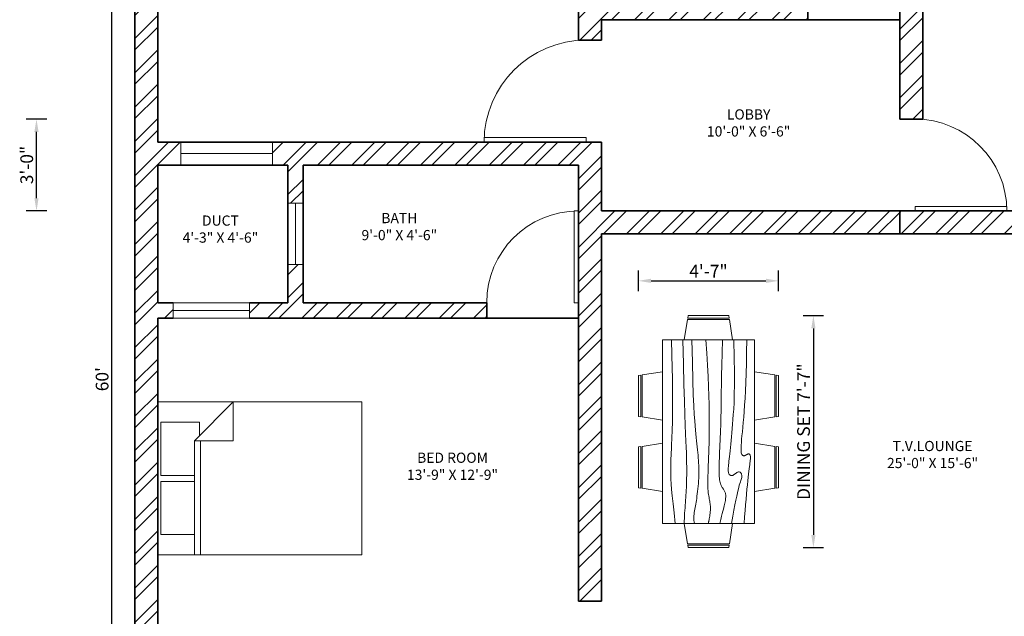
# Model space of a CAD drawing. Units: inches. Extents: x 468 to 1096, y 138 to 946.
# Tile 3 of 6: x 468 to 854, y 448 to 682. Entities that reach past the tile are written whole.
import ezdxf

# ---------------------------------------------------------------- set-up
doc = ezdxf.new("R2010")
doc.units = ezdxf.units.IN
doc.linetypes.add('ACAD_ISO02W100', pattern=[15, 12, -3])
for name, color, linetype, lineweight in [('A-ANNO-DIMS', 2, 'Continuous', 18), ('A-AREA-IDEN', 7, 'Continuous', 18), ('A-DOOR', 3, 'Continuous', 18), ('A-FURN', 8, 'Continuous', 18), ('A-GLAZ', 4, 'Continuous', 18), ('A-WALL', 7, 'Continuous', 35), ('A-WALL-OVHD', 7, 'ACAD_ISO02W100', 18), ('A-WALL-PATT', 8, 'Continuous', 13), ('C-PROP', 7, 'Continuous', 35)]:
    doc.layers.add(name, color=color, linetype=linetype, lineweight=lineweight)
doc.styles.get("Standard").update_dxf_attribs({"font": 'arial.ttf'})
doc.dimstyles.new('ISO-25', dxfattribs={"dimtxt": 5, "dimasz": 5, "dimexe": 4, "dimexo": 4, "dimtad": 1, "dimdec": 1, "dimlunit": 3, "dimtxsty": 'Standard', "dimcen": 2.5, "dimadec": 0, "dimazin": 0, "dimtfac": 1, "dimtdec": 1, "dimtmove": 0, "dimatfit": 3, "dimfxl": 4, "dimfxlon": 1, "dimarcsym": 0})

# ---------------------------------------------------------------- blocks, each defined once
blk = doc.blocks.new('*U2')
for p, q in [((0, 0), (0, -6)), ((40, 0), (40, -6))]:
    blk.add_line(p, q)
blk.add_lwpolyline([(0, 0), (0, 40), (1.75, 40), (1.75, 0)], close=True)
blk.add_arc((0, 0), 40, 0, 90)
blk = doc.blocks.new('*U3')
for p, q in [((0, 0), (0, -6)), ((-36, 0), (-36, -6))]:
    blk.add_line(p, q)
blk.add_lwpolyline([(0, 0), (0, 36), (-1.75, 36), (-1.75, 0)], close=True)
blk.add_arc((0, 0), 36, 90, 180)
blk = doc.blocks.new('Dining Set - 36 x 72 in.')
for p, q in [((-22, 27.5), (-22.1562, 26.50042)), ((-22, 27.5), (-6, 27.5)), ((-5.8437, 26.49966), (-6, 27.5)), ((6, 27.5), (5.8438, 26.50042)), ((6, 27.5), (22, 27.5)), ((22.1563, 26.49966), (22, 27.5)), ((-22.2343, 26.00059), (-23.4847, 17.99762)), ((-22.2304, 26), (-5.7608, 26)), ((-5.8416, 26.5), (-22.1534, 26.5)), ((-4.5152, 17.99762), (-5.7655, 25.99926)), ((5.7657, 26.00059), (4.5153, 17.99762)), ((5.7696, 26), (22.2392, 26)), ((22.1584, 26.5), (5.8466, 26.5)), ((23.4848, 17.99762), (22.2345, 25.99926)), ((36, 18), (-36, 18)), ((-36, 18), (-36, -18)), ((36, -18), (36, 18)), ((-45.5, 8), (-44.5004, 8.15617)), ((-45.5, 8), (-45.5, -8)), ((-44.5, -8.15843), (-44.5, 8.15338)), ((-44.0006, 8.23428), (-35.9976, 9.48474)), ((-44, 8.23041), (-44, -8.23915)), ((44.0006, 8.23428), (35.9976, 9.48474)), ((44, 8.23041), (44, -8.23915)), ((44.5, -8.15843), (44.5, 8.15338)), ((45.5, 8), (44.5005, 8.15617)), ((45.5, 8), (45.5, -8)), ((-44.4997, -8.15631), (-45.5, -8)), ((-35.9976, -9.48476), (-43.9993, -8.2345)), ((35.9976, -9.48476), (43.9993, -8.2345)), ((44.4997, -8.15631), (45.5, -8)), ((-36, -18), (36, -18)), ((-22.2343, -26.0006), (-23.4847, -17.99762)), ((-4.5152, -17.99762), (-5.7655, -25.99928)), ((5.7657, -26.0006), (4.5153, -17.99762)), ((23.4848, -17.99762), (22.2345, -25.99928)), ((-22.2304, -26), (-5.7608, -26)), ((-22, -27.5), (-22.1562, -26.50044)), ((-5.8416, -26.5), (-22.1534, -26.5)), ((-5.8437, -26.49967), (-6, -27.5)), ((5.7696, -26), (22.2392, -26)), ((6, -27.5), (5.8438, -26.50044)), ((22.1584, -26.5), (5.8466, -26.5)), ((22.1563, -26.49967), (22, -27.5)), ((-22, -27.5), (-6, -27.5)), ((6, -27.5), (22, -27.5))]:
    blk.add_line(p, q)
for points in [[(-36, 15), (-31.1772, 14.97754), (-26.8079, 14.91406), (-22.8538, 14.81543), (-19.276, 14.6875), (-16.0362, 14.53613), (-13.0957, 14.36718), (-10.4159, 14.18652), (-7.9583, 14), (-5.6904, 13.81315), (-3.6035, 13.63021), (-1.6954, 13.45508), (0.0365, 13.29166), (1.5945, 13.14388), (2.9811, 13.01562), (4.1988, 12.9108), (5.25, 12.83333), (6.1393, 12.78613), (6.8802, 12.76823), (7.4883, 12.77767), (7.9792, 12.8125), (8.3685, 12.87077), (8.6719, 12.95052), (8.9049, 13.0498), (9.0833, 13.16666), (9.2205, 13.29899), (9.3216, 13.44401), (9.3895, 13.59879), (9.4271, 13.76041), (9.4373, 13.92594), (9.4232, 14.09245), (9.3875, 14.257), (9.3333, 14.41666), (9.2638, 14.56917), (9.1836, 14.71484), (9.0975, 14.85465), (9.0104, 14.98958), (8.9272, 15.1206), (8.8529, 15.2487), (8.7922, 15.37483), (8.75, 15.5), (8.7305, 15.62467), (8.7344, 15.74739), (8.7617, 15.86621), (8.8125, 15.97916), (8.8867, 16.08431), (8.9844, 16.17968), (9.1055, 16.26334), (9.25, 16.33333), (9.4189, 16.38802), (9.6172, 16.42708), (9.8506, 16.45052), (10.125, 16.45833), (10.4463, 16.45052), (10.8203, 16.42708), (11.2529, 16.38802), (11.75, 16.33333), (12.3184, 16.26318), (12.9694, 16.17838), (13.7151, 16.07991), (14.5677, 15.96875), (15.5395, 15.84586), (16.6426, 15.71224), (17.8893, 15.56884), (19.2917, 15.41666), (20.859, 15.25667), (22.5879, 15.08984), (24.4721, 14.91715), (26.5052, 14.73958), (28.6809, 14.5581), (30.9929, 14.3737), (33.4347, 14.18733), (36, 14)], [(-36, 10), (-28.9766, 10.14274), (-23.1725, 10.20442), (-18.4241, 10.19775), (-14.5677, 10.13541), (-11.4399, 10.03011), (-8.877, 9.89453), (-6.7154, 9.74137), (-4.7917, 9.58333), (-2.9698, 9.43082), (-1.2246, 9.28515), (0.4415, 9.14534), (2.026, 9.01041), (3.5266, 8.87939), (4.9408, 8.7513), (6.266, 8.62516), (7.5, 8.5), (8.6411, 8.37549), (9.6914, 8.2539), (10.6538, 8.13818), (11.5312, 8.03125), (12.3267, 7.93603), (13.043, 7.85547), (13.6831, 7.79248), (14.25, 7.75), (14.7471, 7.7303), (15.1797, 7.73307), (15.5537, 7.75732), (15.875, 7.80208), (16.1494, 7.86637), (16.3828, 7.94922), (16.5811, 8.04964), (16.75, 8.16666), (16.8944, 8.29915), (17.0143, 8.44531), (17.1089, 8.60319), (17.1771, 8.77083), (17.218, 8.94629), (17.2305, 9.1276), (17.2137, 9.31282), (17.1667, 9.5), (17.0895, 9.6875), (16.987, 9.875), (16.8649, 10.0625), (16.7292, 10.25), (16.5856, 10.4375), (16.4401, 10.625), (16.2985, 10.8125), (16.1667, 11), (16.05, 11.18733), (15.9518, 11.3737), (15.8752, 11.5581), (15.8229, 11.73958), (15.798, 11.91715), (15.8034, 12.08984), (15.842, 12.25667), (15.9167, 12.41666), (16.0295, 12.56836), (16.1784, 12.70833), (16.3605, 12.83268), (16.5729, 12.9375), (16.8127, 13.01888), (17.0768, 13.07291), (17.3625, 13.0957), (17.6667, 13.08333), (17.9894, 13.03312), (18.3418, 12.94726), (18.7382, 12.82918), (19.1927, 12.68229), (19.7195, 12.51001), (20.3327, 12.31575), (21.0465, 12.10294), (21.875, 11.875), (22.8357, 11.63354), (23.959, 11.37304), (25.2786, 11.08618), (26.8282, 10.76562), (28.6414, 10.40405), (30.752, 9.99414), (33.1936, 9.52856), (36, 9)], [(-36, 5.5), (-30.7157, 5.3348), (-26.069, 5.20963), (-21.9946, 5.11767), (-18.4271, 5.05208), (-15.3009, 5.00602), (-12.5508, 4.97265), (-10.1112, 4.94515), (-7.9167, 4.91666), (-5.909, 4.88167), (-4.0586, 4.83984), (-2.3429, 4.79215), (-0.7396, 4.73958), (0.7739, 4.6831), (2.22, 4.6237), (3.6213, 4.56233), (5, 4.5), (6.373, 4.43782), (7.7344, 4.3776), (9.0723, 4.32129), (10.375, 4.27083), (11.6309, 4.22819), (12.8281, 4.19531), (13.9551, 4.17415), (15, 4.16666), (15.954, 4.17448), (16.819, 4.19791), (17.6001, 4.23698), (18.3021, 4.29166), (18.9299, 4.36198), (19.4883, 4.44791), (19.9823, 4.54948), (20.4167, 4.66666), (20.7969, 4.79899), (21.1302, 4.94401), (21.4245, 5.09879), (21.6875, 5.26041), (21.9271, 5.42594), (22.1511, 5.59245), (22.3672, 5.757), (22.5834, 5.91666), (22.8065, 6.06868), (23.0404, 6.21093), (23.2879, 6.34147), (23.5521, 6.45833), (23.8358, 6.55957), (24.142, 6.64323), (24.4735, 6.70735), (24.8334, 6.75), (25.2235, 6.76969), (25.642, 6.76692), (26.0858, 6.74267), (26.5521, 6.69791), (27.0379, 6.63362), (27.5404, 6.55078), (28.0565, 6.45036), (28.5834, 6.33333), (29.1242, 6.19987), (29.7071, 6.04687), (30.3661, 5.87044), (31.1354, 5.66666), (32.0493, 5.43164), (33.142, 5.16146), (34.4475, 4.85221), (36, 4.5)], [(-36, -1), (-30.7915, -0.6591), (-26.0195, -0.38216), (-21.6519, -0.16284), (-17.6563, 0.00521), (-14.0005, 0.12833), (-10.6523, 0.21289), (-7.5796, 0.26522), (-4.75, 0.29166), (-2.134, 0.29793), (0.2878, 0.28711), (2.5317, 0.26163), (4.6146, 0.22396), (6.5529, 0.17651), (8.3633, 0.12174), (10.0623, 0.06209), (11.6667, 0), (13.1899, -0.06201), (14.6341, -0.1211), (15.9982, -0.17432), (17.2813, -0.21875), (18.4823, -0.25147), (19.6003, -0.26953), (20.6343, -0.27002), (21.5834, -0.25), (22.4481, -0.20768), (23.2357, -0.14584), (23.9549, -0.06836), (24.6146, 0.02083), (25.2235, 0.11784), (25.7904, 0.21875), (26.3241, 0.31966), (26.8334, 0.41666), (27.3265, 0.50618), (27.8099, 0.58593), (28.2894, 0.65397), (28.7709, 0.70833), (29.2601, 0.74707), (29.763, 0.76823), (30.2855, 0.76985), (30.8334, 0.75), (31.4088, 0.70784), (31.9994, 0.64713), (32.589, 0.57275), (33.1615, 0.48958), (33.7008, 0.4025), (34.1908, 0.3164), (34.6153, 0.23616), (34.9584, 0.16666), (35.2099, 0.11165), (35.3848, 0.07031), (35.504, 0.04069), (35.5886, 0.02083), (35.6594, 0.00879), (35.7377, 0.0026), (35.8442, 0.00032), (36, 0)], [(-36, -6.5), (-27.1843, -6.31267), (-20.084, -6.1263), (-14.469, -5.9419), (-10.1094, -5.76042), (-6.7752, -5.58285), (-4.2363, -5.41016), (-2.2629, -5.24333), (-0.625, -5.08334), (0.8708, -4.93099), (2.2715, -4.78646), (3.5872, -4.64974), (4.8281, -4.52084), (6.0046, -4.39974), (7.127, -4.28646), (8.2053, -4.18099), (9.25, -4.08334), (10.2705, -3.99382), (11.2734, -3.91407), (12.2647, -3.84603), (13.25, -3.79167), (14.2354, -3.75293), (15.2266, -3.73177), (16.2295, -3.73015), (17.25, -3.75), (18.2912, -3.79248), (19.3451, -3.85547), (20.4009, -3.93604), (21.4479, -4.03125), (22.4754, -4.13819), (23.4727, -4.25391), (24.4289, -4.37549), (25.3334, -4.5), (26.1785, -4.62492), (26.9694, -4.74935), (27.7145, -4.87281), (28.4219, -4.99479), (29.1, -5.11483), (29.7572, -5.23242), (30.4016, -5.34709), (31.0417, -5.45834), (31.6837, -5.56437), (32.3262, -5.65821), (32.9658, -5.73153), (33.599, -5.77604), (34.2224, -5.78345), (34.8327, -5.74545), (35.4264, -5.65373), (36, -5.5)], [(-36, -10), (-26.4022, -9.81299), (-18.4675, -9.62891), (-11.9839, -9.45069), (-6.7396, -9.28125), (-2.5226, -9.12354), (0.8789, -8.98047), (3.6769, -8.85498), (6.0833, -8.75), (8.2767, -8.66765), (10.3021, -8.60677), (12.1712, -8.56543), (13.8958, -8.54167), (15.4876, -8.53353), (16.9583, -8.53907), (18.3197, -8.55632), (19.5834, -8.58334), (20.7616, -8.61841), (21.8685, -8.66081), (22.9188, -8.71004), (23.9271, -8.76563), (24.9081, -8.82707), (25.8763, -8.89388), (26.8465, -8.96558), (27.8334, -9.04167), (28.8474, -9.12118), (29.8828, -9.20117), (30.93, -9.27824), (31.9792, -9.34896), (33.0205, -9.40991), (34.0443, -9.45768), (35.0407, -9.48885), (36, -9.5)], [(-36, -14.5), (-30.0881, -14.33513), (-25.0332, -14.21224), (-20.7312, -14.12647), (-17.0781, -14.07292), (-13.97, -14.04671), (-11.3027, -14.04297), (-8.9724, -14.05681), (-6.875, -14.08334), (-4.9224, -14.11833), (-3.0905, -14.16016), (-1.3709, -14.20785), (0.2448, -14.26042), (1.7647, -14.3169), (3.1973, -14.3763), (4.5507, -14.43767), (5.8333, -14.5), (7.0554, -14.5621), (8.235, -14.62175), (9.3922, -14.67652), (10.5469, -14.72396), (11.7192, -14.76164), (12.929, -14.78711), (14.1965, -14.79794), (15.5417, -14.79167), (16.9933, -14.76424), (18.6152, -14.70508), (20.4804, -14.60197), (22.6615, -14.44271), (25.2312, -14.21509), (28.2624, -13.9069), (31.8277, -13.50594), (36, -13)]]:
    blk.add_lwpolyline(points)
blk = doc.blocks.new('Bed - Queen')
for p, q in [((0, -80.00003), (0, 0)), ((0, 0), (59.99999, 0)), ((59.99999, 0), (59.99999, -80.00003)), ((7.99999, -1.2), (28.79998, -1.2)), ((7.99999, -14.4), (7.99999, -1.2)), ((28.79998, -1.2), (28.79998, -14.4)), ((31.19999, -1.2), (51.99999, -1.2)), ((31.19999, -14.4), (31.19999, -1.2)), ((51.99999, -1.2), (51.99999, -16.4)), ((0, -14.4), (44.8, -14.4)), ((59.99999, -29.6), (44.8, -14.4)), ((44.8, -14.4), (44.8, -29.6)), ((44.8, -16.8), (0, -16.8)), ((51.99999, -16.4), (46.79936, -16.4)), ((44.8, -29.6), (59.99999, -29.6)), ((59.99999, -80.00003), (0, -80.00003))]:
    blk.add_line(p, q)
blk = doc.blocks.new('*D18')
at = {"layer": 'A-ANNO-DIMS', "color": 0, "lineweight": -2, "transparency": 16777216}
for p, q in [((508.14, 901.16), (500.14, 901.16)), ((504.14, 186.16), (504.14, 896.16)), ((508.14, 181.16), (500.14, 181.16))]:
    blk.add_line(p, q, dxfattribs=at)
at = {"layer": 'A-ANNO-DIMS', "color": 0, "transparency": 16777216}
for points in [[(503.3, 896.16), (504.97, 896.16), (504.14, 901.16)], [(503.3, 186.16), (504.97, 186.16), (504.14, 181.16)]]:
    blk.add_solid(points, dxfattribs=at)
at = {"layer": 'Defpoints', "color": 0, "transparency": 16777216}
for p in [(504.14, 901.16), (513.13, 901.16), (513.13, 181.16)]:
    blk.add_point(p, dxfattribs=at)
at = {"layer": 'A-ANNO-DIMS', "color": 0, "transparency": 16777216, "insert": (500.96, 541.16), "char_height": 5, "attachment_point": 5, "rotation": 90}
blk.add_mtext("60'", dxfattribs=at)
blk = doc.blocks.new('WIN-36-W9')
for p, q in [((0, 9), (0, 0)), ((36, 9), (36, 0)), ((0, 4.5), (36, 4.5))]:
    blk.add_line(p, q)
blk = doc.blocks.new('*D47')
at = {"layer": 'A-ANNO-DIMS', "color": 0, "lineweight": -2, "transparency": 16777216}
for p, q in [((775.26, 566.09), (783.26, 566.09)), ((779.26, 561.09), (779.26, 480.09)), ((775.26, 475.09), (783.26, 475.09))]:
    blk.add_line(p, q, dxfattribs=at)
at = {"layer": 'A-ANNO-DIMS', "color": 0, "transparency": 16777216}
for points in [[(778.42, 561.09), (780.09, 561.09), (779.26, 566.09)], [(778.42, 480.09), (780.09, 480.09), (779.26, 475.09)]]:
    blk.add_solid(points, dxfattribs=at)
at = {"layer": 'Defpoints', "color": 0, "transparency": 16777216}
for p in [(765.61, 566.09), (765.61, 475.09), (779.26, 475.09)]:
    blk.add_point(p, dxfattribs=at)
at = {"layer": 'A-ANNO-DIMS', "color": 0, "transparency": 16777216, "insert": (776.05, 520.59), "char_height": 5, "attachment_point": 5, "rotation": 90}
blk.add_mtext('DINING SET 7\'-7"', dxfattribs=at)
blk = doc.blocks.new('*D48')
at = {"layer": 'A-ANNO-DIMS', "color": 0, "lineweight": -2, "transparency": 16777216}
for p, q in [((710.61, 575.74), (710.61, 583.74)), ((765.61, 575.74), (765.61, 583.74)), ((715.61, 579.74), (760.61, 579.74))]:
    blk.add_line(p, q, dxfattribs=at)
at = {"layer": 'A-ANNO-DIMS', "color": 0, "transparency": 16777216}
for points in [[(715.61, 580.57), (715.61, 578.91), (710.61, 579.74)], [(760.61, 580.57), (760.61, 578.91), (765.61, 579.74)]]:
    blk.add_solid(points, dxfattribs=at)
at = {"layer": 'Defpoints', "color": 0, "transparency": 16777216}
for p in [(765.61, 579.74), (710.61, 566.09), (765.61, 566.09)]:
    blk.add_point(p, dxfattribs=at)
at = {"layer": 'A-ANNO-DIMS', "color": 0, "transparency": 16777216, "insert": (738.11, 582.87), "char_height": 5, "attachment_point": 5}
blk.add_mtext('4\'-7"', dxfattribs=at)
blk = doc.blocks.new('*D61')
at = {"layer": 'A-ANNO-DIMS', "color": 0, "lineweight": -2, "transparency": 16777216}
for p, q in [((594.13, 146.61), (594.13, 138.61)), ((630.13, 146.61), (630.13, 138.61)), ((599.13, 142.61), (625.13, 142.61))]:
    blk.add_line(p, q, dxfattribs=at)
at = {"layer": 'A-ANNO-DIMS', "color": 0, "transparency": 16777216}
for points in [[(599.13, 143.44), (599.13, 141.78), (594.13, 142.61)], [(625.13, 143.44), (625.13, 141.78), (630.13, 142.61)]]:
    blk.add_solid(points, dxfattribs=at)
at = {"layer": 'Defpoints', "color": 0, "transparency": 16777216}
for p in [(594.13, 829.16), (630.13, 826.16), (630.13, 142.61)]:
    blk.add_point(p, dxfattribs=at)
at = {"layer": 'A-ANNO-DIMS', "color": 0, "transparency": 16777216, "insert": (612.13, 145.79), "char_height": 5, "attachment_point": 5}
blk.add_mtext('3\'-0"', dxfattribs=at)
blk = doc.blocks.new('*D63')
at = {"layer": 'A-ANNO-DIMS', "color": 0, "lineweight": -2, "transparency": 16777216}
for p, q in [((777.13, 146.61), (777.13, 138.61)), ((813.13, 146.61), (813.13, 138.61)), ((782.13, 142.61), (808.13, 142.61))]:
    blk.add_line(p, q, dxfattribs=at)
at = {"layer": 'A-ANNO-DIMS', "color": 0, "transparency": 16777216}
for points in [[(782.13, 143.44), (782.13, 141.78), (777.13, 142.61)], [(808.13, 143.44), (808.13, 141.78), (813.13, 142.61)]]:
    blk.add_solid(points, dxfattribs=at)
at = {"layer": 'Defpoints', "color": 0, "transparency": 16777216}
for p in [(777.13, 682.16), (813.13, 682.16), (813.13, 142.61)]:
    blk.add_point(p, dxfattribs=at)
at = {"layer": 'A-ANNO-DIMS', "color": 0, "transparency": 16777216, "insert": (795.13, 145.79), "char_height": 5, "attachment_point": 5}
blk.add_mtext('3\'-0"', dxfattribs=at)
blk = doc.blocks.new('*D66')
at = {"layer": 'A-ANNO-DIMS', "color": 0, "lineweight": -2, "transparency": 16777216}
for p, q in [((696.13, 146.61), (696.13, 138.61)), ((714.39, 146.61), (714.39, 138.61)), ((701.13, 142.61), (709.39, 142.61)), ((714.39, 142.61), (745.11, 142.61))]:
    blk.add_line(p, q, dxfattribs=at)
at = {"layer": 'A-ANNO-DIMS', "color": 0, "transparency": 16777216}
for points in [[(701.13, 143.44), (701.13, 141.78), (696.13, 142.61)], [(709.39, 143.44), (709.39, 141.78), (714.39, 142.61)]]:
    blk.add_solid(points, dxfattribs=at)
at = {"layer": 'Defpoints', "color": 0, "transparency": 16777216}
for p in [(696.13, 820.16), (714.39, 802.16), (714.39, 142.61)]:
    blk.add_point(p, dxfattribs=at)
at = {"layer": 'A-ANNO-DIMS', "color": 0, "transparency": 16777216, "insert": (732.25, 145.82), "char_height": 5, "attachment_point": 5}
blk.add_mtext('1\'-6 1/2"', dxfattribs=at)
blk = doc.blocks.new('*D75')
at = {"layer": 'A-ANNO-DIMS', "color": 0, "lineweight": -2, "transparency": 16777216}
for p, q in [((696.13, 935.71), (696.13, 943.71)), ((736.13, 935.71), (736.13, 943.71)), ((701.13, 939.71), (731.13, 939.71))]:
    blk.add_line(p, q, dxfattribs=at)
at = {"layer": 'A-ANNO-DIMS', "color": 0, "transparency": 16777216}
for points in [[(701.13, 940.54), (701.13, 938.88), (696.13, 939.71)], [(731.13, 940.54), (731.13, 938.88), (736.13, 939.71)]]:
    blk.add_solid(points, dxfattribs=at)
at = {"layer": 'Defpoints', "color": 0, "transparency": 16777216}
for p in [(736.13, 939.71), (696.13, 412.16), (736.13, 412.16)]:
    blk.add_point(p, dxfattribs=at)
at = {"layer": 'A-ANNO-DIMS', "color": 0, "transparency": 16777216, "insert": (716.13, 942.89), "char_height": 5, "attachment_point": 5}
blk.add_mtext('3\'-4"', dxfattribs=at)
blk = doc.blocks.new('*D76')
at = {"layer": 'A-ANNO-DIMS', "color": 0, "lineweight": -2, "transparency": 16777216}
for p, q in [((1087.68, 454.16), (1095.68, 454.16)), ((1091.68, 423.16), (1091.68, 449.16)), ((1087.68, 418.16), (1095.68, 418.16))]:
    blk.add_line(p, q, dxfattribs=at)
at = {"layer": 'A-ANNO-DIMS', "color": 0, "transparency": 16777216}
for points in [[(1090.85, 449.16), (1092.51, 449.16), (1091.68, 454.16)], [(1090.85, 423.16), (1092.51, 423.16), (1091.68, 418.16)]]:
    blk.add_solid(points, dxfattribs=at)
at = {"layer": 'Defpoints', "color": 0, "transparency": 16777216}
for p in [(687.13, 454.16), (1091.68, 454.16), (687.13, 418.16)]:
    blk.add_point(p, dxfattribs=at)
at = {"layer": 'A-ANNO-DIMS', "color": 0, "transparency": 16777216, "insert": (1088.5, 436.16), "char_height": 5, "attachment_point": 5, "rotation": 90}
blk.add_mtext('3\'-0"', dxfattribs=at)
blk = doc.blocks.new('*D77')
at = {"layer": 'A-ANNO-DIMS', "color": 0, "lineweight": -2, "transparency": 16777216}
for p, q in [((651.13, 146.61), (651.13, 138.61)), ((687.13, 146.61), (687.13, 138.61)), ((656.13, 142.61), (682.13, 142.61))]:
    blk.add_line(p, q, dxfattribs=at)
at = {"layer": 'A-ANNO-DIMS', "color": 0, "transparency": 16777216}
for points in [[(656.13, 143.44), (656.13, 141.78), (651.13, 142.61)], [(682.13, 143.44), (682.13, 141.78), (687.13, 142.61)]]:
    blk.add_solid(points, dxfattribs=at)
at = {"layer": 'Defpoints', "color": 0, "transparency": 16777216}
for p in [(651.13, 565.16), (687.13, 565.16), (687.13, 142.61)]:
    blk.add_point(p, dxfattribs=at)
at = {"layer": 'A-ANNO-DIMS', "color": 0, "transparency": 16777216, "insert": (669.13, 145.79), "char_height": 5, "attachment_point": 5}
blk.add_mtext('3\'-0"', dxfattribs=at)
blk = doc.blocks.new('*D78')
at = {"layer": 'A-ANNO-DIMS', "color": 0, "lineweight": -2, "transparency": 16777216}
for p, q in [((573.13, 935.71), (573.13, 943.71)), ((603.13, 935.71), (603.13, 943.71)), ((578.13, 939.71), (598.13, 939.71))]:
    blk.add_line(p, q, dxfattribs=at)
at = {"layer": 'A-ANNO-DIMS', "color": 0, "transparency": 16777216}
for points in [[(578.13, 940.54), (578.13, 938.88), (573.13, 939.71)], [(598.13, 940.54), (598.13, 938.88), (603.13, 939.71)]]:
    blk.add_solid(points, dxfattribs=at)
at = {"layer": 'Defpoints', "color": 0, "transparency": 16777216}
for p in [(603.13, 939.71), (573.13, 250.16), (603.13, 250.16)]:
    blk.add_point(p, dxfattribs=at)
at = {"layer": 'A-ANNO-DIMS', "color": 0, "transparency": 16777216, "insert": (588.13, 942.89), "char_height": 5, "attachment_point": 5}
blk.add_mtext('2\'-6"', dxfattribs=at)
blk = doc.blocks.new('*D79')
at = {"layer": 'A-ANNO-DIMS', "color": 0, "lineweight": -2, "transparency": 16777216}
for p, q in [((612.13, 935.71), (612.13, 943.71)), ((636.13, 935.71), (636.13, 943.71)), ((617.13, 939.71), (631.13, 939.71))]:
    blk.add_line(p, q, dxfattribs=at)
at = {"layer": 'A-ANNO-DIMS', "color": 0, "transparency": 16777216}
for points in [[(617.13, 940.54), (617.13, 938.88), (612.13, 939.71)], [(631.13, 940.54), (631.13, 938.88), (636.13, 939.71)]]:
    blk.add_solid(points, dxfattribs=at)
at = {"layer": 'Defpoints', "color": 0, "transparency": 16777216}
for p in [(636.13, 939.71), (612.13, 241.16), (636.13, 241.16)]:
    blk.add_point(p, dxfattribs=at)
at = {"layer": 'A-ANNO-DIMS', "color": 0, "transparency": 16777216, "insert": (624.13, 942.89), "char_height": 5, "attachment_point": 5}
blk.add_mtext('2\'-0"', dxfattribs=at)
blk = doc.blocks.new('*D80')
at = {"layer": 'A-ANNO-DIMS', "color": 0, "lineweight": -2, "transparency": 16777216}
for p, q in [((684.13, 935.71), (684.13, 943.71)), ((708.13, 935.71), (708.13, 943.71)), ((689.13, 939.71), (703.13, 939.71))]:
    blk.add_line(p, q, dxfattribs=at)
at = {"layer": 'A-ANNO-DIMS', "color": 0, "transparency": 16777216}
for points in [[(689.13, 940.54), (689.13, 938.88), (684.13, 939.71)], [(703.13, 940.54), (703.13, 938.88), (708.13, 939.71)]]:
    blk.add_solid(points, dxfattribs=at)
at = {"layer": 'Defpoints', "color": 0, "transparency": 16777216}
for p in [(708.13, 939.71), (684.13, 250.16), (708.13, 250.16)]:
    blk.add_point(p, dxfattribs=at)
at = {"layer": 'A-ANNO-DIMS', "color": 0, "transparency": 16777216, "insert": (696.13, 942.89), "char_height": 5, "attachment_point": 5}
blk.add_mtext('2\'-0"', dxfattribs=at)
blk = doc.blocks.new('*D81')
at = {"layer": 'A-ANNO-DIMS', "color": 0, "lineweight": -2, "transparency": 16777216}
for p, q in [((708.13, 935.71), (708.13, 943.71)), ((744.13, 935.71), (744.13, 943.71)), ((713.13, 939.71), (739.13, 939.71))]:
    blk.add_line(p, q, dxfattribs=at)
at = {"layer": 'A-ANNO-DIMS', "color": 0, "transparency": 16777216}
for points in [[(713.13, 940.54), (713.13, 938.88), (708.13, 939.71)], [(739.13, 940.54), (739.13, 938.88), (744.13, 939.71)]]:
    blk.add_solid(points, dxfattribs=at)
at = {"layer": 'Defpoints', "color": 0, "transparency": 16777216}
for p in [(744.13, 939.71), (708.13, 250.16), (744.13, 250.16)]:
    blk.add_point(p, dxfattribs=at)
at = {"layer": 'A-ANNO-DIMS', "color": 0, "transparency": 16777216, "insert": (726.13, 942.89), "char_height": 5, "attachment_point": 5}
blk.add_mtext('3\'-0"', dxfattribs=at)
blk = doc.blocks.new('*D82')
at = {"layer": 'A-ANNO-DIMS', "color": 0, "lineweight": -2, "transparency": 16777216}
for p, q in [((1087.68, 674.16), (1095.68, 674.16)), ((1091.68, 639.16), (1091.68, 669.16)), ((1087.68, 634.16), (1095.68, 634.16))]:
    blk.add_line(p, q, dxfattribs=at)
at = {"layer": 'A-ANNO-DIMS', "color": 0, "transparency": 16777216}
for points in [[(1090.85, 669.16), (1092.51, 669.16), (1091.68, 674.16)], [(1090.85, 639.16), (1092.51, 639.16), (1091.68, 634.16)]]:
    blk.add_solid(points, dxfattribs=at)
at = {"layer": 'Defpoints', "color": 0, "transparency": 16777216}
for p in [(687.13, 674.16), (1091.68, 674.16), (687.13, 634.16)]:
    blk.add_point(p, dxfattribs=at)
at = {"layer": 'A-ANNO-DIMS', "color": 0, "transparency": 16777216, "insert": (1088.5, 654.16), "char_height": 5, "attachment_point": 5, "rotation": 90}
blk.add_mtext('3\'-4"', dxfattribs=at)
blk = doc.blocks.new('*D83')
at = {"layer": 'A-ANNO-DIMS', "color": 0, "lineweight": -2, "transparency": 16777216}
for p, q in [((478.58, 643.16), (470.58, 643.16)), ((474.58, 612.16), (474.58, 638.16)), ((478.58, 607.16), (470.58, 607.16))]:
    blk.add_line(p, q, dxfattribs=at)
at = {"layer": 'A-ANNO-DIMS', "color": 0, "transparency": 16777216}
for points in [[(473.75, 638.16), (475.41, 638.16), (474.58, 643.16)], [(473.75, 612.16), (475.41, 612.16), (474.58, 607.16)]]:
    blk.add_solid(points, dxfattribs=at)
at = {"layer": 'Defpoints', "color": 0, "transparency": 16777216}
for p in [(474.58, 643.16), (813.13, 643.16), (813.13, 607.16)]:
    blk.add_point(p, dxfattribs=at)
at = {"layer": 'A-ANNO-DIMS', "color": 0, "transparency": 16777216, "insert": (471.4, 625.16), "char_height": 5, "attachment_point": 5, "rotation": 90}
blk.add_mtext('3\'-0"', dxfattribs=at)
blk = doc.blocks.new('*D85')
at = {"layer": 'A-ANNO-DIMS', "color": 0, "lineweight": -2, "transparency": 16777216}
for p, q in [((528.13, 146.61), (528.13, 138.61)), ((558.13, 146.61), (558.13, 138.61)), ((533.13, 142.61), (553.13, 142.61))]:
    blk.add_line(p, q, dxfattribs=at)
at = {"layer": 'A-ANNO-DIMS', "color": 0, "transparency": 16777216}
for points in [[(533.13, 143.44), (533.13, 141.78), (528.13, 142.61)], [(553.13, 143.44), (553.13, 141.78), (558.13, 142.61)]]:
    blk.add_solid(points, dxfattribs=at)
at = {"layer": 'Defpoints', "color": 0, "transparency": 16777216}
for p in [(528.13, 565.16), (558.13, 565.16), (558.13, 142.61)]:
    blk.add_point(p, dxfattribs=at)
at = {"layer": 'A-ANNO-DIMS', "color": 0, "transparency": 16777216, "insert": (543.13, 145.79), "char_height": 5, "attachment_point": 5}
blk.add_mtext('2\'-6"', dxfattribs=at)
blk = doc.blocks.new('*D86')
at = {"layer": 'A-ANNO-DIMS', "color": 0, "lineweight": -2, "transparency": 16777216}
for p, q in [((1087.68, 610.16), (1095.68, 610.16)), ((1091.68, 591.16), (1091.68, 605.16)), ((1087.68, 586.16), (1095.68, 586.16))]:
    blk.add_line(p, q, dxfattribs=at)
at = {"layer": 'A-ANNO-DIMS', "color": 0, "transparency": 16777216}
for points in [[(1090.85, 605.16), (1092.51, 605.16), (1091.68, 610.16)], [(1090.85, 591.16), (1092.51, 591.16), (1091.68, 586.16)]]:
    blk.add_solid(points, dxfattribs=at)
at = {"layer": 'Defpoints', "color": 0, "transparency": 16777216}
for p in [(579.13, 610.16), (1091.68, 610.16), (579.13, 586.16)]:
    blk.add_point(p, dxfattribs=at)
at = {"layer": 'A-ANNO-DIMS', "color": 0, "transparency": 16777216, "insert": (1088.5, 598.16), "char_height": 5, "attachment_point": 5, "rotation": 90}
blk.add_mtext('2\'-0"', dxfattribs=at)

msp = doc.modelspace()

# ---------------------------------------------------------------- hatches: boundary and pattern name
at = {"layer": 'A-WALL-PATT'}
h = msp.add_hatch(dxfattribs=at)
h.set_pattern_fill('ANSI32', color=256)
h.paths.add_polyline_path([(639.13, 901.16), (513.13, 901.16), (513.13, 181.16), (612.13, 181.16), (612.13, 202.16), (603.13, 202.16), (603.13, 190.16), (522.13, 190.16), (522.13, 241.16), (573.13, 241.16), (573.13, 250.16), (522.13, 250.16), (522.13, 403.16), (696.13, 403.16), (696.13, 418.16), (687.13, 418.16), (687.13, 412.16), (615.37, 412.16), (615.37, 436.16), (611.37, 436.16), (611.37, 412.16), (522.13, 412.16), (522.13, 436.16), (522.13, 565.16), (528.13, 565.16), (528.13, 571.16), (522.13, 571.16), (522.13, 625.16), (531.13, 625.16), (531.13, 634.16), (522.13, 634.16), (522.13, 820.16), (590.13, 820.16), (590.13, 796.16), (594.13, 796.16), (594.13, 820.16), (594.13, 826.16), (594.13, 829.16), (522.13, 829.16), (522.13, 892.16), (630.13, 892.16), (630.13, 872.66), (639.13, 872.66)])
h = msp.add_hatch(dxfattribs=at)
h.set_pattern_fill('ANSI32', color=256)
h.paths.add_polyline_path([(696.13, 634.16), (687.13, 634.16), (650.13, 634.16), (567.13, 634.16), (567.13, 625.16), (573.13, 625.16), (573.13, 610.16), (579.13, 610.16), (579.13, 625.16), (687.13, 625.16), (687.13, 454.16), (696.13, 454.16), (696.13, 598.16), (813.13, 598.16), (813.13, 607.16), (696.13, 607.16)])
h.paths.add_polyline_path([(777.13, 688.16), (777.13, 691.16), (696.13, 691.16), (696.13, 820.16), (721.13, 820.16), (721.13, 829.16), (687.13, 829.16), (687.13, 820.16), (687.13, 674.16), (696.13, 674.16), (696.13, 682.16), (777.13, 682.16)])
h.paths.add_polyline_path([(854.13, 775.16), (822.13, 775.16), (822.13, 835.16), (884.13, 835.16), (884.13, 803.19), (888.13, 803.19), (888.13, 835.16), (987.13, 835.16), (987.13, 817.16), (996.13, 817.16), (996.13, 844.16), (987.13, 844.16), (813.13, 844.16), (813.13, 829.16), (813.13, 823.16), (813.13, 791.16), (813.13, 691.16), (813.13, 688.16), (813.13, 682.16), (813.13, 643.16), (819.13, 643.16), (822.13, 643.16), (822.13, 691.16), (822.13, 766.16), (854.13, 766.16)])
h.paths.add_polyline_path([(996.13, 775.16), (996.13, 784.16), (996.13, 793.16), (987.13, 793.16), (987.13, 775.16), (884.13, 775.16), (884.13, 766.16), (987.13, 766.16), (987.13, 718.16), (996.13, 718.16)], flags=17)
h.paths.add_polyline_path([(781.13, 829.16), (757.13, 829.16), (757.13, 820.16), (781.13, 820.16)])
h = msp.add_hatch(dxfattribs=at)
h.set_pattern_fill('ANSI32', color=256)
h.paths.add_polyline_path([(1053.13, 412.16), (1044.13, 412.16), (1044.13, 241.16), (1053.13, 241.16)])
h.paths.add_polyline_path([(996.13, 448.16), (987.13, 448.16), (987.13, 412.16), (942.13, 412.16), (942.13, 403.16), (996.13, 403.16)])
h.paths.add_polyline_path([(996.13, 532.16), (987.13, 532.16), (987.13, 496.16), (996.13, 496.16)])
h.paths.add_polyline_path([(996.13, 646.16), (987.13, 646.16), (987.13, 607.16), (813.13, 607.16), (813.13, 598.16), (822.13, 598.16), (987.13, 598.16), (987.13, 592.16), (996.13, 592.16), (996.13, 598.16), (996.13, 607.16)])
h.paths.add_polyline_path([(894.13, 412.16), (849.13, 412.16), (849.13, 403.16), (894.13, 403.16)])
h.paths.add_polyline_path([(801.13, 412.16), (744.13, 412.16), (744.13, 250.16), (744.13, 241.16), (777.13, 241.16), (777.13, 250.16), (753.13, 250.16), (753.13, 403.16), (801.13, 403.16)])
h.paths.add_polyline_path([(744.13, 412.16), (736.13, 412.16), (736.13, 403.16), (744.13, 403.16)])
h = msp.add_hatch(dxfattribs=at)
h.set_pattern_fill('ANSI32', color=256)
h.paths.add_polyline_path([(651.13, 571.16), (579.13, 571.16), (579.13, 586.16), (573.13, 586.16), (573.13, 571.16), (558.13, 571.16), (558.13, 565.16), (573.13, 565.16), (651.13, 565.16)])

# ---------------------------------------------------------------- linework, layer by layer
at = {"layer": 'A-GLAZ'}
for p, q in [((573.13, 610.16), (579.13, 610.16)), ((576.13, 586.16), (576.13, 610.16)), ((573.13, 586.16), (579.13, 586.16)), ((528.13, 571.16), (528.13, 565.16)), ((528.13, 571.16), (558.13, 571.16)), ((528.13, 568.16), (558.13, 568.16)), ((558.13, 571.16), (558.13, 565.16)), ((528.13, 565.16), (558.13, 565.16))]:
    msp.add_line(p, q, dxfattribs=at)
at = {"layer": 'A-WALL'}
for p, q in [((522.13, 820.16), (522.13, 634.16)), ((687.13, 820.16), (687.13, 674.16)), ((777.13, 691.16), (777.13, 682.16)), ((813.13, 691.16), (813.13, 682.16)), ((822.13, 643.16), (822.13, 691.16)), ((813.13, 682.16), (696.13, 682.16)), ((696.13, 682.16), (696.13, 674.16)), ((696.13, 674.16), (687.13, 674.16)), ((822.13, 643.16), (813.13, 643.16)), ((687.13, 634.16), (522.13, 634.16)), ((687.13, 634.16), (696.13, 634.16)), ((696.13, 634.16), (696.13, 607.16)), ((522.13, 625.16), (522.13, 571.16)), ((573.13, 625.16), (522.13, 625.16)), ((573.13, 571.16), (573.13, 625.16)), ((687.13, 625.16), (579.13, 625.16)), ((579.13, 571.16), (579.13, 625.16)), ((687.13, 454.16), (687.13, 625.16)), ((696.13, 607.16), (813.13, 607.16)), ((813.13, 607.16), (813.13, 598.16)), ((987.13, 607.16), (813.13, 607.16)), ((696.13, 598.16), (696.13, 454.16)), ((696.13, 598.16), (813.13, 598.16)), ((522.13, 571.16), (528.13, 571.16)), ((558.13, 571.16), (573.13, 571.16)), ((579.13, 571.16), (651.13, 571.16)), ((651.13, 571.16), (651.13, 565.16)), ((522.13, 565.16), (528.13, 565.16)), ((522.13, 565.16), (522.13, 412.16)), ((558.13, 565.16), (573.13, 565.16)), ((687.13, 565.16), (573.13, 565.16)), ((687.13, 454.16), (696.13, 454.16))]:
    msp.add_line(p, q, dxfattribs=at)
for points in [[(813.13, 643.16), (813.13, 682.16)], [(987.13, 598.16), (822.13, 598.16), (813.13, 598.16)]]:
    msp.add_lwpolyline(points, dxfattribs=at)
at = {"layer": 'A-WALL-OVHD', "ltscale": 0.6}
for p, q in [((813.13, 607.16), (696.13, 607.16)), ((813.13, 598.16), (696.13, 598.16))]:
    msp.add_line(p, q, dxfattribs=at)
at = {"layer": 'C-PROP'}
msp.add_line((513.13, 901.16), (513.13, 181.16), dxfattribs=at)

# ---------------------------------------------------------------- block references
at = {"layer": 'A-DOOR'}
for name, p, rotation in [('*U2', (690.13, 634.16), 90), ('*U3', (819.13, 607.16), 270)]:
    msp.add_blockref(name, p, dxfattribs=dict(at, rotation=rotation))
msp.add_blockref('*U3', (687.13, 571.16), dxfattribs=at)
at = {"layer": 'A-FURN'}
for name, p, rotation in [('Dining Set - 36 x 72 in.', (738.11, 520.59), 270), ('Bed - Queen', (522.13, 472.25), 90)]:
    msp.add_blockref(name, p, dxfattribs=dict(at, rotation=rotation))
at = {"layer": 'A-GLAZ', "rotation": 180}
msp.add_blockref('WIN-36-W9', (567.13, 634.16), dxfattribs=at)

# ---------------------------------------------------------------- texts
at = {"layer": 'A-AREA-IDEN', "char_height": 4, "attachment_point": 1}
for s, insert in [('\\pxqc;LOBBY\\P10\'-0" X 6\'-6"', (735.73, 647.01)), ('\\pxqc;BATH\\P9\'-0" X 4\'-6"', (598.75, 606.35)), ('\\pxqc;DUCT\\P4\'-3" X 4\'-6"', (528.58, 605.37)), ('\\pxqc;T.V.LOUNGE\\P25\'-0" X 15\'-6"', (807.86, 516.95)), ('\\pxqc;BED ROOM\\P13\'-9" X 12\'-9"', (619.6, 512.35))]:
    msp.add_mtext_dynamic_manual_height_columns(s, width=36.2598, gutter_width=12.5, heights=[0], dxfattribs=dict(at, insert=insert))

# ---------------------------------------------------------------- dimensions: what is measured, and where the dimension line sits
at = {"layer": 'A-ANNO-DIMS'}
for base, p1, p2, picture, middle in [((603.13, 939.71), (573.13, 250.16), (603.13, 250.16), '*D78', (588.13, 942.89)), ((636.13, 939.71), (612.13, 241.16), (636.13, 241.16), '*D79', (624.13, 942.89)), ((708.13, 939.71), (684.13, 250.16), (708.13, 250.16), '*D80', (696.13, 942.89)), ((736.13, 939.71), (696.13, 412.16), (736.13, 412.16), '*D75', (716.13, 942.89)), ((744.13, 939.71), (708.13, 250.16), (744.13, 250.16), '*D81', (726.13, 942.89)), ((630.13, 142.61), (594.13, 829.16), (630.13, 826.16), '*D61', (612.13, 145.79)), ((714.39, 142.61), (696.13, 820.16), (714.39, 802.16), '*D66', (732.25, 145.82)), ((813.13, 142.61), (777.13, 682.16), (813.13, 682.16), '*D63', (795.13, 145.79)), ((765.61, 579.74), (710.61, 566.09), (765.61, 566.09), '*D48', (738.11, 582.87)), ((558.13, 142.61), (528.13, 565.16), (558.13, 565.16), '*D85', (543.13, 145.79)), ((687.13, 142.61), (651.13, 565.16), (687.13, 565.16), '*D77', (669.13, 145.79))]:
    dim = msp.add_linear_dim(base=base, p1=p1, p2=p2, dimstyle='ISO-25', override={"dimdec": 1, "dimlfac": 1, "dimrnd": 0, "dimzin": 1, "dimdsep": 46, "dimlunit": 4, "dimfrac": 2}, dxfattribs=at)
    dim.commit()
    dim.dimension.update_dxf_attribs({"geometry": picture, "text_midpoint": middle})
for base, p1, p2, override, picture, middle in [((504.14, 901.16), (513.13, 181.16), (513.13, 901.16), {"dimclrd": 0, "dimclre": 0, "dimclrt": 0}, '*D18', (500.96, 541.16)), ((1091.68, 674.16), (687.13, 634.16), (687.13, 674.16), {"dimdec": 1, "dimlfac": 1, "dimrnd": 0, "dimzin": 1, "dimdsep": 46, "dimlunit": 4, "dimfrac": 2}, '*D82', (1088.5, 654.16)), ((474.58, 643.16), (813.13, 607.16), (813.13, 643.16), {"dimdec": 1, "dimlfac": 1, "dimrnd": 0, "dimzin": 1, "dimdsep": 46, "dimlunit": 4, "dimfrac": 2}, '*D83', (471.4, 625.16)), ((1091.68, 610.16), (579.13, 586.16), (579.13, 610.16), {"dimdec": 1, "dimlfac": 1, "dimrnd": 0, "dimzin": 1, "dimdsep": 46, "dimlunit": 4, "dimfrac": 2}, '*D86', (1088.5, 598.16)), ((1091.68, 454.16), (687.13, 418.16), (687.13, 454.16), {"dimdec": 1, "dimlfac": 1, "dimrnd": 0, "dimzin": 1, "dimdsep": 46, "dimlunit": 4, "dimfrac": 2}, '*D76', (1088.5, 436.16))]:
    dim = msp.add_linear_dim(base=base, p1=p1, p2=p2, angle=90, dimstyle='ISO-25', override=override, dxfattribs=at)
    dim.commit()
    dim.dimension.update_dxf_attribs({"geometry": picture, "text_midpoint": middle})
dim = msp.add_linear_dim(base=(779.26, 475.09), p1=(765.61, 566.09), p2=(765.61, 475.09), angle=270, text='DINING SET <>', dimstyle='ISO-25', override={"dimdec": 1, "dimlfac": 1, "dimrnd": 0, "dimzin": 1, "dimdsep": 46, "dimlunit": 4, "dimfrac": 2}, dxfattribs=at)
dim.commit()
dim.dimension.update_dxf_attribs({"geometry": '*D47', "text_midpoint": (776.05, 520.59)})

doc.saveas('drawing.dxf')
